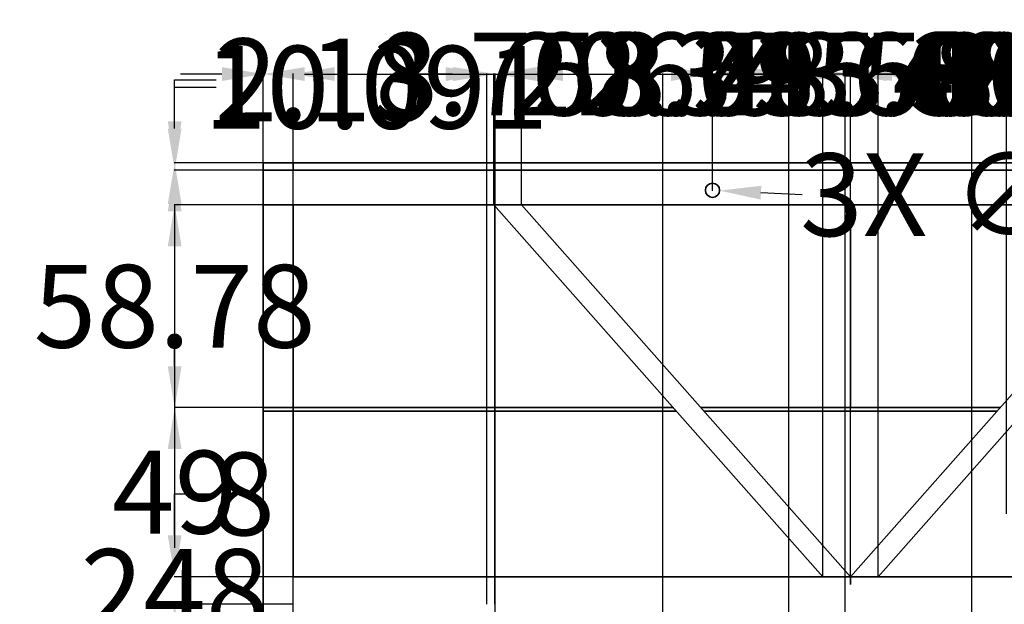
# Model space of a CAD drawing. Units: inches. Extents: x 172 to 828, y 190 to 777.
# Tile 3 of 9: x 188 to 474, y 607 to 777. Entities that reach past the tile are written whole.
import ezdxf

# ---------------------------------------------------------------- set-up
doc = ezdxf.new("R2010")
doc.units = ezdxf.units.IN
doc.header["$MEASUREMENT"] = 0
doc.layers.add('A-ANNO-DIMS', color=2, linetype='Continuous', lineweight=18)
doc.layers.add('A-ELEV', color=7, linetype='Continuous', lineweight=35)
doc.styles.get("Standard").update_dxf_attribs({"font": 'arial.ttf'})
doc.dimstyles.get("Standard").update_dxf_attribs({"dimtxt": 24, "dimasz": 12, "dimexe": 0.18, "dimexo": 0.0625, "dimgap": 0.09, "dimtad": 0, "dimtih": 1, "dimtoh": 1, "dimdec": 0, "dimzin": 0, "dimdsep": 46, "dimlunit": 3, "dimtxsty": 'Standard', "dimcen": 0.09, "dimadec": 0, "dimazin": 0, "dimtfac": 1, "dimtdec": 0, "dimtofl": 0, "dimtmove": 0, "dimatfit": 3, "dimfxl": 1, "dimtolj": 1, "dimtzin": 0, "dimarcsym": 0})

# ---------------------------------------------------------------- blocks, each defined once
blk = doc.blocks.new('*D6')
at = {"layer": 'A-ANNO-DIMS', "color": 0, "lineweight": -2, "transparency": 16777216}
for p, q in [((411.3, 579.39), (424.02, 579.39)), ((423.84, 567.39), (423.84, 549.9)), ((423.84, 507.39), (423.84, 524.88)), ((411.3, 495.39), (424.02, 495.39))]:
    blk.add_line(p, q, dxfattribs=at)
at = {"layer": 'A-ANNO-DIMS', "color": 0, "transparency": 16777216}
for points in [[(421.84, 567.39), (425.84, 567.39), (423.84, 579.39)], [(421.84, 507.39), (425.84, 507.39), (423.84, 495.39)]]:
    blk.add_solid(points, dxfattribs=at)
at = {"layer": 'Defpoints', "color": 0, "transparency": 16777216}
for p in [(411.24, 579.39), (423.84, 579.39), (411.24, 495.39)]:
    blk.add_point(p, dxfattribs=at)
at = {"layer": 'A-ANNO-DIMS', "color": 0, "transparency": 16777216, "insert": (423.84, 537.39), "char_height": 24, "attachment_point": 5}
blk.add_mtext('\\A1;GLAZED DOUBLE DOOR 84 TYP.', dxfattribs=at)
blk = doc.blocks.new('*D10')
at = {"layer": 'A-ANNO-DIMS', "color": 0, "lineweight": -2, "transparency": 16777216}
for p, q in [((258.78, 231.45), (258.78, 761.27)), ((270.78, 761.09), (412.23, 761.09)), ((606.78, 761.09), (465.33, 761.09)), ((618.78, 735.45), (618.78, 761.27))]:
    blk.add_line(p, q, dxfattribs=at)
at = {"layer": 'A-ANNO-DIMS', "color": 0, "transparency": 16777216}
for points in [[(270.78, 763.09), (270.78, 759.09), (258.78, 761.09)], [(606.78, 763.09), (606.78, 759.09), (618.78, 761.09)]]:
    blk.add_solid(points, dxfattribs=at)
at = {"layer": 'Defpoints', "color": 0, "transparency": 16777216}
for p in [(618.78, 761.09), (618.78, 735.39), (258.78, 231.39)]:
    blk.add_point(p, dxfattribs=at)
at = {"layer": 'A-ANNO-DIMS', "color": 0, "transparency": 16777216, "insert": (438.78, 761.09), "char_height": 24, "attachment_point": 5}
blk.add_mtext('\\A1;360', dxfattribs=at)
blk = doc.blocks.new('*D14')
at = {"layer": 'A-ANNO-DIMS', "color": 0, "lineweight": -2, "transparency": 16777216}
for p, q in [((258.72, 735.39), (232.9, 735.39)), ((233.08, 723.39), (233.08, 623.74)), ((233.08, 499.39), (233.08, 599.05)), ((258.72, 487.39), (232.9, 487.39))]:
    blk.add_line(p, q, dxfattribs=at)
at = {"layer": 'A-ANNO-DIMS', "color": 0, "transparency": 16777216}
for points in [[(231.08, 723.39), (235.08, 723.39), (233.08, 735.39)], [(231.08, 499.39), (235.08, 499.39), (233.08, 487.39)]]:
    blk.add_solid(points, dxfattribs=at)
at = {"layer": 'Defpoints', "color": 0, "transparency": 16777216}
for p in [(233.08, 735.39), (258.78, 735.39), (258.78, 487.39)]:
    blk.add_point(p, dxfattribs=at)
at = {"layer": 'A-ANNO-DIMS', "color": 0, "transparency": 16777216, "insert": (233.08, 611.39), "char_height": 24, "attachment_point": 5}
blk.add_mtext('\\A1;248', dxfattribs=at)
blk = doc.blocks.new('*D36')
at = {"layer": 'A-ANNO-DIMS', "color": 0, "lineweight": -2, "transparency": 16777216}
for p, q in [((258.78, 735.45), (258.78, 761.27)), ((270.78, 761.09), (412.23, 761.09)), ((606.78, 761.09), (465.33, 761.09)), ((618.78, 735.45), (618.78, 761.27))]:
    blk.add_line(p, q, dxfattribs=at)
at = {"layer": 'A-ANNO-DIMS', "color": 0, "transparency": 16777216}
for points in [[(270.78, 763.09), (270.78, 759.09), (258.78, 761.09)], [(606.78, 763.09), (606.78, 759.09), (618.78, 761.09)]]:
    blk.add_solid(points, dxfattribs=at)
at = {"layer": 'Defpoints', "color": 0, "transparency": 16777216}
for p in [(618.78, 761.09), (258.78, 735.39), (618.78, 735.39)]:
    blk.add_point(p, dxfattribs=at)
at = {"layer": 'A-ANNO-DIMS', "color": 0, "transparency": 16777216, "insert": (438.78, 761.09), "char_height": 24, "attachment_point": 5}
blk.add_mtext('\\A1;360', dxfattribs=at)
blk = doc.blocks.new('*D37')
at = {"layer": 'A-ANNO-DIMS', "color": 0, "lineweight": -2, "transparency": 16777216}
for p, q in [((258.72, 664.39), (232.9, 664.39)), ((233.08, 652.39), (233.08, 652.24)), ((233.08, 627.39), (233.08, 627.55)), ((267.42, 615.39), (232.9, 615.39))]:
    blk.add_line(p, q, dxfattribs=at)
at = {"layer": 'A-ANNO-DIMS', "color": 0, "transparency": 16777216}
for points in [[(231.08, 652.39), (235.08, 652.39), (233.08, 664.39)], [(231.08, 627.39), (235.08, 627.39), (233.08, 615.39)]]:
    blk.add_solid(points, dxfattribs=at)
at = {"layer": 'Defpoints', "color": 0, "transparency": 16777216}
for p in [(233.08, 664.39), (258.78, 664.39), (267.48, 615.39)]:
    blk.add_point(p, dxfattribs=at)
at = {"layer": 'A-ANNO-DIMS', "color": 0, "transparency": 16777216, "insert": (233.08, 639.89), "char_height": 24, "attachment_point": 5}
blk.add_mtext('\\A1;49', dxfattribs=at)
blk = doc.blocks.new('*D38')
at = {"layer": 'A-ANNO-DIMS', "color": 0, "lineweight": -2, "transparency": 16777216}
for p, q in [((258.72, 723.17), (232.9, 723.17)), ((233.08, 711.17), (233.08, 706.12)), ((233.08, 676.39), (233.08, 681.44)), ((258.72, 664.39), (232.9, 664.39))]:
    blk.add_line(p, q, dxfattribs=at)
at = {"layer": 'A-ANNO-DIMS', "color": 0, "transparency": 16777216}
for points in [[(231.08, 711.17), (235.08, 711.17), (233.08, 723.17)], [(231.08, 676.39), (235.08, 676.39), (233.08, 664.39)]]:
    blk.add_solid(points, dxfattribs=at)
at = {"layer": 'Defpoints', "color": 0, "transparency": 16777216}
for p in [(233.08, 723.17), (258.78, 723.17), (258.78, 664.39)]:
    blk.add_point(p, dxfattribs=at)
at = {"layer": 'A-ANNO-DIMS', "color": 0, "transparency": 16777216, "insert": (233.08, 693.78), "char_height": 24, "attachment_point": 5}
blk.add_mtext('\\A1;58.78', dxfattribs=at)
blk = doc.blocks.new('*D39')
at = {"layer": 'A-ANNO-DIMS', "color": 0, "lineweight": -2, "transparency": 16777216}
for p, q in [((233.08, 745.26), (233.08, 757.26)), ((233.08, 757.26), (245.08, 757.26)), ((258.72, 733.26), (232.9, 733.26)), ((258.72, 723.17), (232.9, 723.17)), ((233.08, 711.17), (233.08, 699.17))]:
    blk.add_line(p, q, dxfattribs=at)
at = {"layer": 'A-ANNO-DIMS', "color": 0, "transparency": 16777216}
for points in [[(231.08, 745.26), (235.08, 745.26), (233.08, 733.26)], [(231.08, 711.17), (235.08, 711.17), (233.08, 723.17)]]:
    blk.add_solid(points, dxfattribs=at)
at = {"layer": 'Defpoints', "color": 0, "transparency": 16777216}
for p in [(233.08, 733.26), (258.78, 733.26), (258.78, 723.17)]:
    blk.add_point(p, dxfattribs=at)
at = {"layer": 'A-ANNO-DIMS', "color": 0, "transparency": 16777216, "insert": (291.54, 757.26), "char_height": 24, "attachment_point": 5}
blk.add_mtext('\\A1;10.091', dxfattribs=at)
blk = doc.blocks.new('*D40')
at = {"layer": 'A-ANNO-DIMS', "color": 0, "lineweight": -2, "transparency": 16777216}
for p, q in [((233.08, 747.39), (233.08, 759.39)), ((233.08, 759.39), (245.08, 759.39)), ((258.72, 735.39), (232.9, 735.39)), ((258.72, 733.26), (232.9, 733.26)), ((233.08, 721.26), (233.08, 709.26))]:
    blk.add_line(p, q, dxfattribs=at)
at = {"layer": 'A-ANNO-DIMS', "color": 0, "transparency": 16777216}
for points in [[(231.08, 747.39), (235.08, 747.39), (233.08, 735.39)], [(231.08, 721.26), (235.08, 721.26), (233.08, 733.26)]]:
    blk.add_solid(points, dxfattribs=at)
at = {"layer": 'Defpoints', "color": 0, "transparency": 16777216}
for p in [(233.08, 735.39), (258.78, 735.39), (258.78, 733.26)]:
    blk.add_point(p, dxfattribs=at)
at = {"layer": 'A-ANNO-DIMS', "color": 0, "transparency": 16777216, "insert": (276.54, 759.39), "char_height": 24, "attachment_point": 5}
blk.add_mtext('\\A1;2.13', dxfattribs=at)
blk = doc.blocks.new('*D41')
at = {"layer": 'A-ANNO-DIMS', "color": 0, "lineweight": -2, "transparency": 16777216}
for p, q in [((246.78, 761.09), (234.78, 761.09)), ((258.78, 723.23), (258.78, 761.27)), ((267.48, 723.23), (267.48, 761.27)), ((279.48, 761.09), (291.48, 761.09))]:
    blk.add_line(p, q, dxfattribs=at)
at = {"layer": 'A-ANNO-DIMS', "color": 0, "transparency": 16777216}
for points in [[(246.78, 763.09), (246.78, 759.09), (258.78, 761.09)], [(279.48, 763.09), (279.48, 759.09), (267.48, 761.09)]]:
    blk.add_solid(points, dxfattribs=at)
at = {"layer": 'Defpoints', "color": 0, "transparency": 16777216}
for p in [(267.48, 761.09), (258.78, 723.17), (267.48, 723.17)]:
    blk.add_point(p, dxfattribs=at)
at = {"layer": 'A-ANNO-DIMS', "color": 0, "transparency": 16777216, "insert": (332.08, 761.09), "char_height": 24, "attachment_point": 5}
blk.add_mtext('\\A1;8.703', dxfattribs=at)
blk = doc.blocks.new('*D42')
at = {"layer": 'A-ANNO-DIMS', "color": 0, "lineweight": -2, "transparency": 16777216}
for p, q in [((267.48, 723.23), (267.48, 761.27)), ((279.48, 761.09), (313.71, 761.09)), ((325.71, 723.23), (325.71, 761.27)), ((325.71, 761.09), (337.71, 761.09))]:
    blk.add_line(p, q, dxfattribs=at)
at = {"layer": 'A-ANNO-DIMS', "color": 0, "transparency": 16777216}
for points in [[(279.48, 763.09), (279.48, 759.09), (267.48, 761.09)], [(313.71, 763.09), (313.71, 759.09), (325.71, 761.09)]]:
    blk.add_solid(points, dxfattribs=at)
at = {"layer": 'Defpoints', "color": 0, "transparency": 16777216}
for p in [(325.71, 761.09), (267.48, 723.17), (325.71, 723.17)]:
    blk.add_point(p, dxfattribs=at)
at = {"layer": 'A-ANNO-DIMS', "color": 0, "transparency": 16777216, "insert": (378.29, 761.09), "char_height": 24, "attachment_point": 5}
blk.add_mtext('\\A1;58.23', dxfattribs=at)
blk = doc.blocks.new('*D43')
at = {"layer": 'A-ANNO-DIMS', "color": 0, "lineweight": -2, "transparency": 16777216}
for p, q in [((313.71, 761.09), (301.71, 761.09)), ((325.71, 723.23), (325.71, 761.27)), ((333.72, 723.23), (333.72, 761.27)), ((345.72, 761.09), (357.72, 761.09))]:
    blk.add_line(p, q, dxfattribs=at)
at = {"layer": 'A-ANNO-DIMS', "color": 0, "transparency": 16777216}
for points in [[(313.71, 763.09), (313.71, 759.09), (325.71, 761.09)], [(345.72, 763.09), (345.72, 759.09), (333.72, 761.09)]]:
    blk.add_solid(points, dxfattribs=at)
at = {"layer": 'Defpoints', "color": 0, "transparency": 16777216}
for p in [(333.72, 761.09), (325.71, 723.17), (333.72, 723.17)]:
    blk.add_point(p, dxfattribs=at)
at = {"layer": 'A-ANNO-DIMS', "color": 0, "transparency": 16777216, "insert": (398.32, 761.09), "char_height": 24, "attachment_point": 5}
blk.add_mtext('\\A1;8.013', dxfattribs=at)
blk = doc.blocks.new('*D44')
at = {"layer": 'A-ANNO-DIMS', "color": 0, "lineweight": -2, "transparency": 16777216}
for p, q in [((333.72, 723.23), (333.72, 761.27)), ((345.72, 761.09), (377.1, 761.09)), ((389.1, 727.47), (389.1, 761.27)), ((389.1, 761.09), (401.1, 761.09))]:
    blk.add_line(p, q, dxfattribs=at)
at = {"layer": 'A-ANNO-DIMS', "color": 0, "transparency": 16777216}
for points in [[(345.72, 763.09), (345.72, 759.09), (333.72, 761.09)], [(377.1, 763.09), (377.1, 759.09), (389.1, 761.09)]]:
    blk.add_solid(points, dxfattribs=at)
at = {"layer": 'Defpoints', "color": 0, "transparency": 16777216}
for p in [(389.1, 761.09), (389.1, 727.4), (333.72, 723.17)]:
    blk.add_point(p, dxfattribs=at)
at = {"layer": 'A-ANNO-DIMS', "color": 0, "transparency": 16777216, "insert": (441.71, 761.09), "char_height": 24, "attachment_point": 5}
blk.add_mtext('\\A1;55.38', dxfattribs=at)
blk = doc.blocks.new('*D45')
at = {"layer": 'A-ANNO-DIMS', "color": 0, "lineweight": -2, "transparency": 16777216}
for p, q in [((389.1, 727.47), (389.1, 761.27)), ((401.1, 761.09), (417.14, 761.09)), ((429.14, 615.45), (429.14, 761.27)), ((429.14, 761.09), (441.14, 761.09))]:
    blk.add_line(p, q, dxfattribs=at)
at = {"layer": 'A-ANNO-DIMS', "color": 0, "transparency": 16777216}
for points in [[(401.1, 763.09), (401.1, 759.09), (389.1, 761.09)], [(417.14, 763.09), (417.14, 759.09), (429.14, 761.09)]]:
    blk.add_solid(points, dxfattribs=at)
at = {"layer": 'Defpoints', "color": 0, "transparency": 16777216}
for p in [(429.14, 761.09), (389.1, 727.4), (429.14, 615.39)]:
    blk.add_point(p, dxfattribs=at)
at = {"layer": 'A-ANNO-DIMS', "color": 0, "transparency": 16777216, "insert": (482.2, 761.09), "char_height": 24, "attachment_point": 5}
blk.add_mtext('\\A1;40.03', dxfattribs=at)
blk = doc.blocks.new('*D46')
at = {"layer": 'A-ANNO-DIMS', "color": 0, "lineweight": -2, "transparency": 16777216}
for p, q in [((429.14, 615.45), (429.14, 761.27)), ((441.14, 761.09), (445.77, 761.09)), ((485.14, 761.09), (480.51, 761.09)), ((497.14, 727.47), (497.14, 761.27))]:
    blk.add_line(p, q, dxfattribs=at)
at = {"layer": 'A-ANNO-DIMS', "color": 0, "transparency": 16777216}
for points in [[(441.14, 763.09), (441.14, 759.09), (429.14, 761.09)], [(485.14, 763.09), (485.14, 759.09), (497.14, 761.09)]]:
    blk.add_solid(points, dxfattribs=at)
at = {"layer": 'Defpoints', "color": 0, "transparency": 16777216}
for p in [(497.14, 761.09), (497.14, 727.4), (429.14, 615.39)]:
    blk.add_point(p, dxfattribs=at)
at = {"layer": 'A-ANNO-DIMS', "color": 0, "transparency": 16777216, "insert": (463.14, 761.09), "char_height": 24, "attachment_point": 5}
blk.add_mtext('\\A1;68', dxfattribs=at)
blk = doc.blocks.new('*D52')
at = {"layer": 'A-ANNO-DIMS', "color": 0, "lineweight": -2, "transparency": 16777216}
for p, q in [((409.12, 761.09), (397.12, 761.09)), ((421.12, 615.45), (421.12, 761.27)), ((429.14, 615.45), (429.14, 761.27)), ((441.14, 761.09), (453.14, 761.09))]:
    blk.add_line(p, q, dxfattribs=at)
at = {"layer": 'A-ANNO-DIMS', "color": 0, "transparency": 16777216}
for points in [[(409.12, 763.09), (409.12, 759.09), (421.12, 761.09)], [(441.14, 763.09), (441.14, 759.09), (429.14, 761.09)]]:
    blk.add_solid(points, dxfattribs=at)
at = {"layer": 'Defpoints', "color": 0, "transparency": 16777216}
for p in [(429.14, 761.09), (421.12, 615.39), (429.14, 615.39)]:
    blk.add_point(p, dxfattribs=at)
at = {"layer": 'A-ANNO-DIMS', "color": 0, "transparency": 16777216, "insert": (493.74, 761.09), "char_height": 24, "attachment_point": 5}
blk.add_mtext('\\A1;8.013', dxfattribs=at)
blk = doc.blocks.new('*D53')
at = {"layer": 'A-ANNO-DIMS', "color": 0, "lineweight": -2, "transparency": 16777216}
for p, q in [((417.14, 761.09), (405.14, 761.09)), ((429.14, 615.45), (429.14, 761.27)), ((437.15, 615.45), (437.15, 761.27)), ((449.15, 761.09), (461.15, 761.09))]:
    blk.add_line(p, q, dxfattribs=at)
at = {"layer": 'A-ANNO-DIMS', "color": 0, "transparency": 16777216}
for points in [[(417.14, 763.09), (417.14, 759.09), (429.14, 761.09)], [(449.15, 763.09), (449.15, 759.09), (437.15, 761.09)]]:
    blk.add_solid(points, dxfattribs=at)
at = {"layer": 'Defpoints', "color": 0, "transparency": 16777216}
for p in [(437.15, 761.09), (429.14, 615.39), (437.15, 615.39)]:
    blk.add_point(p, dxfattribs=at)
at = {"layer": 'A-ANNO-DIMS', "color": 0, "transparency": 16777216, "insert": (501.75, 761.09), "char_height": 24, "attachment_point": 5}
blk.add_mtext('\\A1;8.013', dxfattribs=at)
blk = doc.blocks.new('*D54')
at = {"layer": 'A-ANNO-DIMS', "color": 0, "lineweight": -2, "transparency": 16777216}
for p, q in [((267.48, 615.45), (267.48, 761.27)), ((279.48, 761.09), (330.13, 761.09)), ((462.39, 761.09), (411.75, 761.09)), ((474.39, 633.61), (474.39, 761.27))]:
    blk.add_line(p, q, dxfattribs=at)
at = {"layer": 'A-ANNO-DIMS', "color": 0, "transparency": 16777216}
for points in [[(279.48, 763.09), (279.48, 759.09), (267.48, 761.09)], [(462.39, 763.09), (462.39, 759.09), (474.39, 761.09)]]:
    blk.add_solid(points, dxfattribs=at)
at = {"layer": 'Defpoints', "color": 0, "transparency": 16777216}
for p in [(474.39, 761.09), (474.39, 633.55), (267.48, 615.39)]:
    blk.add_point(p, dxfattribs=at)
at = {"layer": 'A-ANNO-DIMS', "color": 0, "transparency": 16777216, "insert": (370.94, 761.09), "char_height": 24, "attachment_point": 5}
blk.add_mtext('\\A1;206.9', dxfattribs=at)
blk = doc.blocks.new('*D68')
at = {"layer": 'A-ANNO-DIMS', "color": 0, "lineweight": -2, "transparency": 16777216}
for p, q in [((258.72, 607.39), (232.9, 607.39)), ((233.08, 595.39), (233.08, 559.74)), ((233.08, 499.39), (233.08, 535.05)), ((258.72, 487.39), (232.9, 487.39))]:
    blk.add_line(p, q, dxfattribs=at)
at = {"layer": 'A-ANNO-DIMS', "color": 0, "transparency": 16777216}
for points in [[(231.08, 595.39), (235.08, 595.39), (233.08, 607.39)], [(231.08, 499.39), (235.08, 499.39), (233.08, 487.39)]]:
    blk.add_solid(points, dxfattribs=at)
at = {"layer": 'Defpoints', "color": 0, "transparency": 16777216}
for p in [(233.08, 607.39), (258.78, 607.39), (258.78, 487.39)]:
    blk.add_point(p, dxfattribs=at)
at = {"layer": 'A-ANNO-DIMS', "color": 0, "transparency": 16777216, "insert": (233.08, 547.39), "char_height": 24, "attachment_point": 5}
blk.add_mtext('\\A1;120', dxfattribs=at)
blk = doc.blocks.new('*D69')
at = {"layer": 'A-ANNO-DIMS', "color": 0, "lineweight": -2, "transparency": 16777216}
for p, q in [((233.08, 627.39), (233.08, 639.39)), ((233.08, 639.39), (245.08, 639.39)), ((267.42, 615.39), (232.9, 615.39)), ((258.72, 607.39), (232.9, 607.39)), ((233.08, 595.39), (233.08, 583.39))]:
    blk.add_line(p, q, dxfattribs=at)
at = {"layer": 'A-ANNO-DIMS', "color": 0, "transparency": 16777216}
for points in [[(231.08, 627.39), (235.08, 627.39), (233.08, 615.39)], [(231.08, 595.39), (235.08, 595.39), (233.08, 607.39)]]:
    blk.add_solid(points, dxfattribs=at)
at = {"layer": 'Defpoints', "color": 0, "transparency": 16777216}
for p in [(233.08, 615.39), (267.48, 615.39), (258.78, 607.39)]:
    blk.add_point(p, dxfattribs=at)
at = {"layer": 'A-ANNO-DIMS', "color": 0, "transparency": 16777216, "insert": (253.08, 639.39), "char_height": 24, "attachment_point": 5}
blk.add_mtext('\\A1;8', dxfattribs=at)
blk = doc.blocks.new('*D72')
at = {"layer": 'A-ANNO-DIMS', "color": 0, "lineweight": -2, "transparency": 16777216}
for p, q in [((267.42, 607.39), (232.9, 607.39)), ((233.08, 595.39), (233.08, 583.53)), ((233.08, 547.39), (233.08, 559.25)), ((267.42, 535.39), (232.9, 535.39))]:
    blk.add_line(p, q, dxfattribs=at)
at = {"layer": 'A-ANNO-DIMS', "color": 0, "transparency": 16777216}
for points in [[(231.08, 595.39), (235.08, 595.39), (233.08, 607.39)], [(231.08, 547.39), (235.08, 547.39), (233.08, 535.39)]]:
    blk.add_solid(points, dxfattribs=at)
at = {"layer": 'Defpoints', "color": 0, "transparency": 16777216}
for p in [(233.08, 607.39), (267.48, 607.39), (267.48, 535.39)]:
    blk.add_point(p, dxfattribs=at)
at = {"layer": 'A-ANNO-DIMS', "color": 0, "transparency": 16777216, "insert": (233.08, 571.39), "char_height": 24, "attachment_point": 5}
blk.add_mtext('\\A1;72', dxfattribs=at)
blk = doc.blocks.new('*D73')
at = {"layer": 'A-ANNO-DIMS', "color": 0, "lineweight": -2, "transparency": 16777216}
for p, q in [((246.78, 761.09), (234.78, 761.09)), ((258.78, 607.45), (258.78, 761.27)), ((267.48, 495.45), (267.48, 761.27)), ((279.48, 761.09), (291.48, 761.09))]:
    blk.add_line(p, q, dxfattribs=at)
at = {"layer": 'A-ANNO-DIMS', "color": 0, "transparency": 16777216}
for points in [[(246.78, 763.09), (246.78, 759.09), (258.78, 761.09)], [(279.48, 763.09), (279.48, 759.09), (267.48, 761.09)]]:
    blk.add_solid(points, dxfattribs=at)
at = {"layer": 'Defpoints', "color": 0, "transparency": 16777216}
for p in [(267.48, 761.09), (258.78, 607.39), (267.48, 495.39)]:
    blk.add_point(p, dxfattribs=at)
at = {"layer": 'A-ANNO-DIMS', "color": 0, "transparency": 16777216, "insert": (332.08, 761.09), "char_height": 24, "attachment_point": 5}
blk.add_mtext('\\A1;8.703', dxfattribs=at)
blk = doc.blocks.new('*D74')
at = {"layer": 'A-ANNO-DIMS', "color": 0, "lineweight": -2, "transparency": 16777216}
for p, q in [((267.48, 495.45), (267.48, 761.27)), ((279.48, 761.09), (314.08, 761.09)), ((326.08, 495.45), (326.08, 761.27)), ((326.08, 761.09), (338.08, 761.09))]:
    blk.add_line(p, q, dxfattribs=at)
at = {"layer": 'A-ANNO-DIMS', "color": 0, "transparency": 16777216}
for points in [[(279.48, 763.09), (279.48, 759.09), (267.48, 761.09)], [(314.08, 763.09), (314.08, 759.09), (326.08, 761.09)]]:
    blk.add_solid(points, dxfattribs=at)
at = {"layer": 'Defpoints', "color": 0, "transparency": 16777216}
for p in [(326.08, 761.09), (267.48, 495.39), (326.08, 495.39)]:
    blk.add_point(p, dxfattribs=at)
at = {"layer": 'A-ANNO-DIMS', "color": 0, "transparency": 16777216, "insert": (378.68, 761.09), "char_height": 24, "attachment_point": 5}
blk.add_mtext('\\A1;58.59', dxfattribs=at)
blk = doc.blocks.new('*D75')
at = {"layer": 'A-ANNO-DIMS', "color": 0, "lineweight": -2, "transparency": 16777216}
for p, q in [((326.08, 495.45), (326.08, 761.27)), ((338.08, 761.09), (362.66, 761.09)), ((374.66, 495.45), (374.66, 761.27)), ((374.66, 761.09), (386.66, 761.09))]:
    blk.add_line(p, q, dxfattribs=at)
at = {"layer": 'A-ANNO-DIMS', "color": 0, "transparency": 16777216}
for points in [[(338.08, 763.09), (338.08, 759.09), (326.08, 761.09)], [(362.66, 763.09), (362.66, 759.09), (374.66, 761.09)]]:
    blk.add_solid(points, dxfattribs=at)
at = {"layer": 'Defpoints', "color": 0, "transparency": 16777216}
for p in [(374.66, 761.09), (326.08, 495.39), (374.66, 495.39)]:
    blk.add_point(p, dxfattribs=at)
at = {"layer": 'A-ANNO-DIMS', "color": 0, "transparency": 16777216, "insert": (427.75, 761.09), "char_height": 24, "attachment_point": 5}
blk.add_mtext('\\A1;48.59', dxfattribs=at)
blk = doc.blocks.new('*D76')
at = {"layer": 'A-ANNO-DIMS', "color": 0, "lineweight": -2, "transparency": 16777216}
for p, q in [((399.24, 761.09), (387.24, 761.09)), ((411.24, 495.45), (411.24, 761.27)), ((427.59, 495.45), (427.59, 761.27)), ((439.59, 761.09), (451.59, 761.09))]:
    blk.add_line(p, q, dxfattribs=at)
at = {"layer": 'A-ANNO-DIMS', "color": 0, "transparency": 16777216}
for points in [[(399.24, 763.09), (399.24, 759.09), (411.24, 761.09)], [(439.59, 763.09), (439.59, 759.09), (427.59, 761.09)]]:
    blk.add_solid(points, dxfattribs=at)
at = {"layer": 'Defpoints', "color": 0, "transparency": 16777216}
for p in [(427.59, 761.09), (411.24, 495.39), (427.59, 495.39)]:
    blk.add_point(p, dxfattribs=at)
at = {"layer": 'A-ANNO-DIMS', "color": 0, "transparency": 16777216, "insert": (500.36, 761.09), "char_height": 24, "attachment_point": 5}
blk.add_mtext('\\A1;16.356', dxfattribs=at)
blk = doc.blocks.new('*D77')
at = {"layer": 'A-ANNO-DIMS', "color": 0, "lineweight": -2, "transparency": 16777216}
for p, q in [((427.59, 495.45), (427.59, 761.27)), ((439.59, 761.09), (452.34, 761.09)), ((464.34, 495.45), (464.34, 761.27)), ((464.34, 761.09), (476.34, 761.09))]:
    blk.add_line(p, q, dxfattribs=at)
at = {"layer": 'A-ANNO-DIMS', "color": 0, "transparency": 16777216}
for points in [[(439.59, 763.09), (439.59, 759.09), (427.59, 761.09)], [(452.34, 763.09), (452.34, 759.09), (464.34, 761.09)]]:
    blk.add_solid(points, dxfattribs=at)
at = {"layer": 'Defpoints', "color": 0, "transparency": 16777216}
for p in [(464.34, 761.09), (427.59, 495.39), (464.34, 495.39)]:
    blk.add_point(p, dxfattribs=at)
at = {"layer": 'A-ANNO-DIMS', "color": 0, "transparency": 16777216, "insert": (516.86, 761.09), "char_height": 24, "attachment_point": 5}
blk.add_mtext('\\A1;36.74', dxfattribs=at)
blk = doc.blocks.new('*D78')
at = {"layer": 'A-ANNO-DIMS', "color": 0, "lineweight": -2, "transparency": 16777216}
for p, q in [((452.34, 761.09), (440.34, 761.09)), ((464.34, 607.45), (464.34, 761.27)), ((488.42, 607.45), (488.42, 761.27)), ((500.42, 761.09), (512.42, 761.09))]:
    blk.add_line(p, q, dxfattribs=at)
at = {"layer": 'A-ANNO-DIMS', "color": 0, "transparency": 16777216}
for points in [[(452.34, 763.09), (452.34, 759.09), (464.34, 761.09)], [(500.42, 763.09), (500.42, 759.09), (488.42, 761.09)]]:
    blk.add_solid(points, dxfattribs=at)
at = {"layer": 'Defpoints', "color": 0, "transparency": 16777216}
for p in [(488.42, 761.09), (464.34, 607.39), (488.42, 607.39)]:
    blk.add_point(p, dxfattribs=at)
at = {"layer": 'A-ANNO-DIMS', "color": 0, "transparency": 16777216, "insert": (562.56, 761.09), "char_height": 24, "attachment_point": 5}
blk.add_mtext('\\A1;24.088', dxfattribs=at)
blk = doc.blocks.new('*D79')
at = {"layer": 'A-ANNO-DIMS', "color": 0, "lineweight": -2, "transparency": 16777216}
for p, q in [((476.42, 761.09), (464.42, 761.09)), ((488.42, 607.45), (488.42, 761.27)), ((499.69, 607.45), (499.69, 761.27)), ((511.69, 761.09), (523.69, 761.09))]:
    blk.add_line(p, q, dxfattribs=at)
at = {"layer": 'A-ANNO-DIMS', "color": 0, "transparency": 16777216}
for points in [[(476.42, 763.09), (476.42, 759.09), (488.42, 761.09)], [(511.69, 763.09), (511.69, 759.09), (499.69, 761.09)]]:
    blk.add_solid(points, dxfattribs=at)
at = {"layer": 'Defpoints', "color": 0, "transparency": 16777216}
for p in [(499.69, 761.09), (488.42, 607.39), (499.69, 607.39)]:
    blk.add_point(p, dxfattribs=at)
at = {"layer": 'A-ANNO-DIMS', "color": 0, "transparency": 16777216, "insert": (563.15, 761.09), "char_height": 24, "attachment_point": 5}
blk.add_mtext('\\A1;11.27', dxfattribs=at)
blk = doc.blocks.new('*D87')
at = {"layer": 'A-ANNO-DIMS', "color": 0, "lineweight": -2, "transparency": 16777216}
for p, q in [((311.68, 761.09), (299.68, 761.09)), ((323.68, 607.45), (323.68, 761.27)), ((326.01, 607.45), (326.01, 761.27)), ((338.01, 761.09), (350.01, 761.09))]:
    blk.add_line(p, q, dxfattribs=at)
at = {"layer": 'A-ANNO-DIMS', "color": 0, "transparency": 16777216}
for points in [[(311.68, 763.09), (311.68, 759.09), (323.68, 761.09)], [(338.01, 763.09), (338.01, 759.09), (326.01, 761.09)]]:
    blk.add_solid(points, dxfattribs=at)
at = {"layer": 'Defpoints', "color": 0, "transparency": 16777216}
for p in [(326.01, 761.09), (323.68, 607.39), (326.01, 607.39)]:
    blk.add_point(p, dxfattribs=at)
at = {"layer": 'A-ANNO-DIMS', "color": 0, "transparency": 16777216, "insert": (381.43, 761.09), "char_height": 24, "attachment_point": 5}
blk.add_mtext('\\A1;2.34', dxfattribs=at)
blk = doc.blocks.new('*D92')
at = {"layer": 'A-ANNO-DIMS', "color": 0, "lineweight": -2, "transparency": 16777216}
for p, q in [((389.01, 727.4), (389.19, 727.4)), ((389.1, 727.31), (389.1, 727.49)), ((415.15, 726.11), (403.16, 726.7))]:
    blk.add_line(p, q, dxfattribs=at)
at = {"layer": 'A-ANNO-DIMS', "color": 0, "transparency": 16777216}
blk.add_solid([(403.26, 728.7), (403.06, 724.71), (391.17, 727.3)], dxfattribs=at)
at = {"layer": 'Defpoints', "color": 0, "transparency": 16777216}
for p in [(387.03, 727.51), (391.17, 727.3)]:
    blk.add_point(p, dxfattribs=at)
at = {"layer": 'A-ANNO-DIMS', "color": 0, "transparency": 16777216, "insert": (493.92, 726.11), "char_height": 24, "attachment_point": 5}
blk.add_mtext('\\A1;3X ∅4.147', dxfattribs=at)

msp = doc.modelspace()

# ---------------------------------------------------------------- linework, layer by layer
at = {"layer": 'A-ELEV'}
for p, q in [((258.7792, 487.3923), (258.7792, 735.3923)), ((267.4822, 735.3923), (258.7792, 735.3923)), ((618.7792, 735.3923), (267.4822, 735.3923)), ((267.4822, 733.2598), (267.4822, 735.3923)), ((618.7792, 733.2598), (258.7792, 733.2598)), ((618.7792, 723.1684), (258.7792, 723.1684)), ((267.4822, 615.3923), (267.4822, 723.1684)), ((421.1221, 615.3923), (325.7074, 723.1684)), ((429.1355, 615.3923), (333.7209, 723.1684)), ((429.1355, 615.3923), (524.5502, 723.1684)), ((429.1355, 664.3923), (429.1355, 723.1684)), ((429.1355, 723.1684), (429.1355, 664.3923)), ((437.149, 615.3923), (532.5637, 723.1684)), ((377.7422, 664.3923), (258.7792, 664.3923)), ((378.6275, 663.3923), (258.7792, 663.3923)), ((472.5155, 664.3923), (385.7556, 664.3923)), ((471.6302, 663.3923), (386.6409, 663.3923)), ((606.8158, 615.3923), (267.4822, 615.3923)), ((429.1355, 615.3923), (429.1355, 613.1506))]:
    msp.add_line(p, q, dxfattribs=at)
msp.add_circle((389.104, 727.4027), 2.0735, dxfattribs=at)

# ---------------------------------------------------------------- dimensions: what is measured, and where the dimension line sits
at = {"layer": 'A-ANNO-DIMS'}
for base, p1, p2, override, picture, middle in [((233.0792, 735.3923), (258.7792, 733.2598), (258.7792, 735.3923), {"dimdec": 2, "dimlfac": 1, "dimrnd": 0, "dimzin": 0, "dimdsep": 46, "dimlunit": 2}, '*D40', (276.5443, 759.3923)), ((233.0792, 733.2598), (258.7792, 723.1684), (258.7792, 733.2598), {"dimdec": 3, "dimlfac": 1, "dimrnd": 0, "dimzin": 0, "dimdsep": 46, "dimlunit": 2}, '*D39', (291.5403, 757.2598)), ((233.0792, 735.3923), (258.7792, 487.3923), (258.7792, 735.3923), {"dimdec": 0, "dimlfac": 1, "dimrnd": 0, "dimzin": 0, "dimdsep": 46, "dimlunit": 2}, '*D14', (233.0792, 611.3923)), ((233.0792, 723.1684), (258.7792, 664.3923), (258.7792, 723.1684), {"dimdec": 2, "dimlfac": 1, "dimrnd": 0, "dimzin": 0, "dimdsep": 46, "dimlunit": 2}, '*D38', (233.0792, 693.7803)), ((233.0792, 664.3923), (267.4822, 615.3923), (258.7792, 664.3923), {"dimdec": 0, "dimlfac": 1, "dimrnd": 0, "dimzin": 0, "dimdsep": 46, "dimlunit": 2}, '*D37', (233.0792, 639.8923)), ((233.0792, 615.3923), (258.7792, 607.3923), (267.4822, 615.3923), {"dimdec": 0, "dimlfac": 1, "dimrnd": 0, "dimzin": 0, "dimdsep": 46, "dimlunit": 2}, '*D69', (253.0764, 639.3923)), ((233.0792, 607.3923), (258.7792, 487.3923), (258.7792, 607.3923), {"dimdec": 0, "dimlfac": 1, "dimrnd": 0, "dimzin": 0, "dimdsep": 46, "dimlunit": 2}, '*D68', (233.0792, 547.3923)), ((233.0792, 607.3923), (267.4822, 535.3923), (267.4822, 607.3923), {"dimdec": 0, "dimlfac": 1, "dimrnd": 0, "dimzin": 0, "dimdsep": 46, "dimlunit": 2}, '*D72', (233.0792, 571.3923))]:
    dim = msp.add_linear_dim(base=base, p1=p1, p2=p2, angle=90, dimstyle='Standard', override=override, dxfattribs=at)
    dim.commit()
    dim.dimension.update_dxf_attribs({"geometry": picture, "text_midpoint": middle})
for base, p1, p2, override, picture, middle in [((267.4822, 761.0923), (258.7792, 723.1684), (267.4822, 723.1684), {"dimdec": 3, "dimlfac": 1, "dimrnd": 0, "dimzin": 0, "dimdsep": 46, "dimlunit": 2}, '*D41', (332.0824, 761.0923)), ((267.4822, 761.0923), (258.7792, 607.3923), (267.4822, 495.3923), {"dimdec": 3, "dimlfac": 1, "dimrnd": 0, "dimzin": 0, "dimdsep": 46, "dimlunit": 2}, '*D73', (332.0824, 761.0923)), ((618.7792, 761.0923), (258.7792, 231.3923), (618.7792, 735.3923), {"dimdec": 0, "dimlfac": 1, "dimrnd": 0, "dimzin": 0, "dimdsep": 46, "dimlunit": 2}, '*D10', (438.7792, 761.0923)), ((618.7792, 761.0923), (258.7792, 735.3923), (618.7792, 735.3923), {"dimdec": 0, "dimlfac": 1, "dimrnd": 0, "dimzin": 0, "dimdsep": 46, "dimlunit": 2}, '*D36', (438.7792, 761.0923)), ((325.7074, 761.0923), (267.4822, 723.1684), (325.7074, 723.1684), {"dimdec": 2, "dimlfac": 1, "dimrnd": 0, "dimzin": 0, "dimdsep": 46, "dimlunit": 2}, '*D42', (378.2913, 761.0923)), ((474.3939, 761.0923), (267.4822, 615.3923), (474.3939, 633.5521), {"dimdec": 1, "dimlfac": 1, "dimrnd": 0, "dimzin": 0, "dimdsep": 46, "dimlunit": 2}, '*D54', (370.9381, 761.0923)), ((326.0759, 761.0923), (267.4822, 495.3923), (326.0759, 495.3923), {"dimdec": 2, "dimlfac": 1, "dimrnd": 0, "dimzin": 0, "dimdsep": 46, "dimlunit": 2}, '*D74', (378.6843, 761.0923)), ((326.0147, 761.0923), (323.6783, 607.3923), (326.0147, 607.3923), {"dimdec": 2, "dimlfac": 1, "dimrnd": 0, "dimzin": 0, "dimdsep": 46, "dimlunit": 2}, '*D87', (381.4307, 761.0923)), ((333.72087, 761.09229), (325.70742, 723.16837), (333.72087, 723.16837), {"dimdec": 3, "dimlfac": 1, "dimrnd": 0, "dimzin": 0, "dimdsep": 46, "dimlunit": 2}, '*D43', (398.3211, 761.09229)), ((374.6632, 761.0923), (326.0759, 495.3923), (374.6632, 495.3923), {"dimdec": 2, "dimlfac": 1, "dimrnd": 0, "dimzin": 0, "dimdsep": 46, "dimlunit": 2}, '*D75', (427.7546, 761.0923)), ((389.104, 761.0923), (333.7209, 723.1684), (389.104, 727.4027), {"dimdec": 2, "dimlfac": 1, "dimrnd": 0, "dimzin": 0, "dimdsep": 46, "dimlunit": 2}, '*D44', (441.7124, 761.0923)), ((427.5926, 761.0923), (411.2362, 495.3923), (427.5926, 495.3923), {"dimdec": 3, "dimlfac": 1, "dimrnd": 0, "dimzin": 0, "dimdsep": 46, "dimlunit": 2}, '*D76', (500.362, 761.0923)), ((429.1355, 761.0923), (389.104, 727.4027), (429.1355, 615.3923), {"dimdec": 2, "dimlfac": 1, "dimrnd": 0, "dimzin": 0, "dimdsep": 46, "dimlunit": 2}, '*D45', (482.2024, 761.0923)), ((429.1355, 761.0923), (421.1221, 615.3923), (429.1355, 615.3923), {"dimdec": 3, "dimlfac": 1, "dimrnd": 0, "dimzin": 0, "dimdsep": 46, "dimlunit": 2}, '*D52', (493.7358, 761.0923)), ((437.149, 761.09229), (429.13555, 615.39229), (437.149, 615.39229), {"dimdec": 3, "dimlfac": 1, "dimrnd": 0, "dimzin": 0, "dimdsep": 46, "dimlunit": 2}, '*D53', (501.74924, 761.09229)), ((464.3356, 761.0923), (427.5926, 495.3923), (464.3356, 495.3923), {"dimdec": 2, "dimlfac": 1, "dimrnd": 0, "dimzin": 0, "dimdsep": 46, "dimlunit": 2}, '*D77', (516.8622, 761.0923)), ((497.1421, 761.0923), (429.1355, 615.3923), (497.1421, 727.4027), {"dimdec": 0, "dimlfac": 1, "dimrnd": 0, "dimzin": 0, "dimdsep": 46, "dimlunit": 2}, '*D46', (463.1388, 761.0923)), ((488.4232, 761.0923), (464.3356, 607.3923), (488.4232, 607.3923), {"dimdec": 3, "dimlfac": 1, "dimrnd": 0, "dimzin": 0, "dimdsep": 46, "dimlunit": 2}, '*D78', (562.5596, 761.0923)), ((499.6941, 761.0923), (488.4232, 607.3923), (499.6941, 607.3923), {"dimdec": 2, "dimlfac": 1, "dimrnd": 0, "dimzin": 0, "dimdsep": 46, "dimlunit": 2}, '*D79', (563.1484, 761.0923))]:
    dim = msp.add_linear_dim(base=base, p1=p1, p2=p2, dimstyle='Standard', override=override, dxfattribs=at)
    dim.commit()
    dim.dimension.update_dxf_attribs({"geometry": picture, "text_midpoint": middle})
dim = msp.add_diameter_dim_2p(p1=(387.033, 727.5056), p2=(391.1749, 727.2998), text='3X <>', dimstyle='Standard', override={"dimdec": 3, "dimlfac": 1, "dimrnd": 0, "dimzin": 0, "dimdsep": 46, "dimlunit": 2}, dxfattribs=at)
dim.commit()
dim.dimension.update_dxf_attribs({"geometry": '*D92', "text_midpoint": (415.1453, 726.1083), "dimtype": 163})
dim = msp.add_linear_dim(base=(423.8362, 579.3923), p1=(411.2362, 495.3923), p2=(411.2362, 579.3923), angle=90, text='GLAZED DOUBLE DOOR <> TYP.', dimstyle='Standard', override={"dimdec": 0, "dimlfac": 1, "dimrnd": 0, "dimzin": 0, "dimdsep": 46, "dimlunit": 2}, dxfattribs=at)
dim.commit()
dim.dimension.update_dxf_attribs({"geometry": '*D6', "text_midpoint": (423.8362, 537.3923)})

doc.saveas('drawing.dxf')
